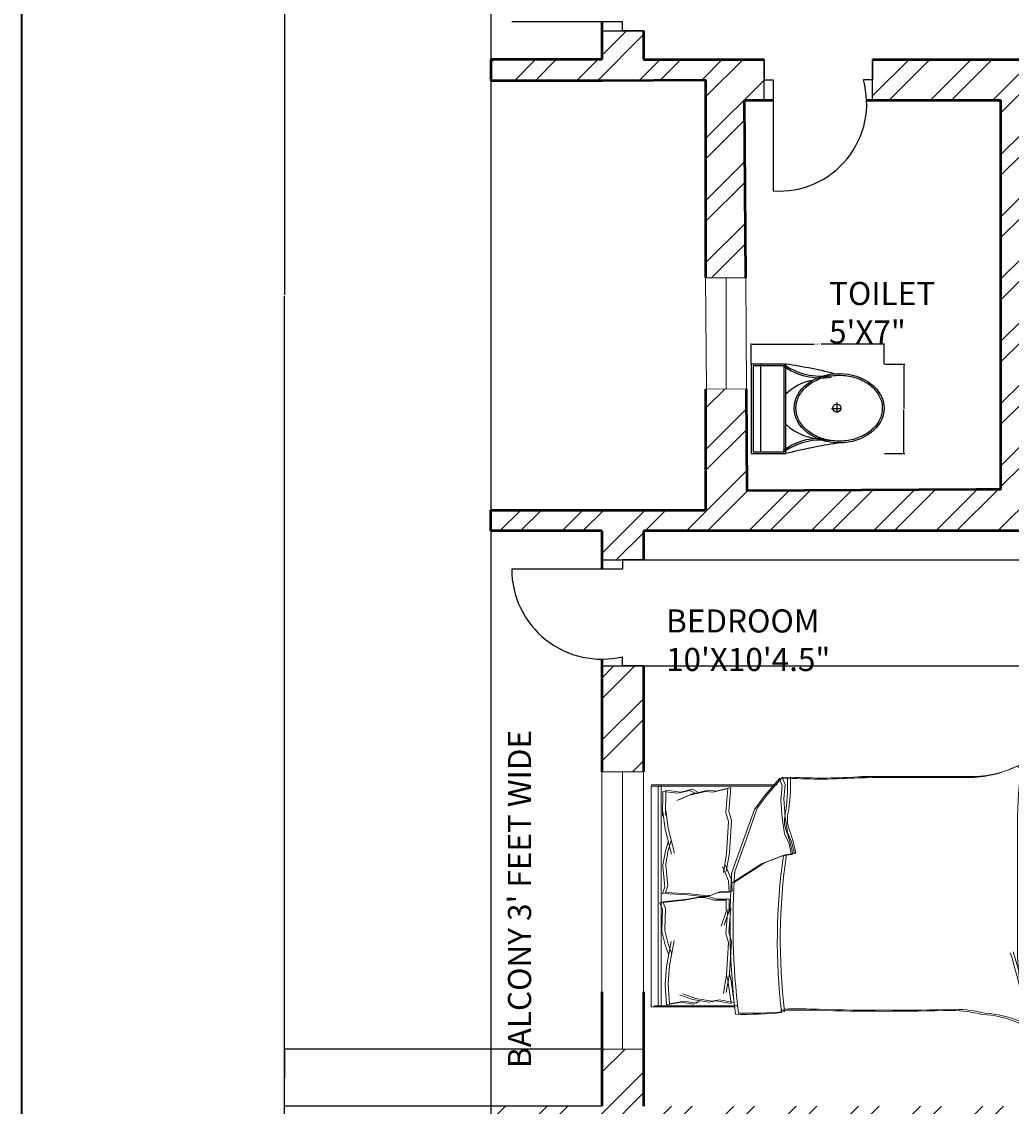
# Model space of a CAD drawing. Units: inches. Extents: x 1980 to 2738, y 1471 to 2568.
# Tile 7 of 22: x 1980 to 2194, y 1878 to 2112. Entities that reach past the tile are written whole.
import ezdxf

# ---------------------------------------------------------------- set-up
doc = ezdxf.new("R2010")
doc.units = ezdxf.units.IN
for name, color, linetype, lineweight in [('A-ANNO-DIMS', 2, 'Continuous', 18), ('A-ANNO-TTLB', 7, 'Continuous', 35), ('A-AREA-IDEN', 7, 'Continuous', 18), ('A-DOOR', 31, 'Continuous', 25), ('A-FLOR-BALC', 7, 'Continuous', 25), ('A-FLOR-FIXT', 8, 'Continuous', 25), ('A-FURN', 8, 'Continuous', 18), ('A-GLAZ', 141, 'Continuous', 18), ('A-WALL', 7, 'Continuous', 50)]:
    doc.layers.add(name, color=color, linetype=linetype, lineweight=lineweight)
doc.layers.add('A-WALL-PATT', color=9, linetype='Continuous', lineweight=13, true_color=0xd19cc7)
doc.styles.get("Standard").update_dxf_attribs({"font": 'arial.ttf'})
doc.dimstyles.get("Standard").update_dxf_attribs({"dimtxt": 0.18, "dimasz": 0.18, "dimexe": 0.18, "dimexo": 0.0625, "dimgap": 0.09, "dimtad": 0, "dimtih": 1, "dimtoh": 1, "dimdec": 4, "dimzin": 0, "dimdsep": 46, "dimtxsty": 'Standard', "dimcen": 0.09, "dimadec": 0, "dimazin": 0, "dimtfac": 1, "dimtdec": 4, "dimtofl": 0, "dimtmove": 0, "dimatfit": 3, "dimfxl": 1, "dimtolj": 1, "dimtzin": 0, "dimarcsym": 0})

# ---------------------------------------------------------------- blocks, each defined once
blk = doc.blocks.new('A$C31115884')
for p, q in [((257.5, 466.4), (257.5, 523.2)), ((283.1, 497.7), (223.4, 497.7)), ((0, 200), (0, 0)), ((520, 200), (0, 200)), ((10, 190), (10, 10)), ((510, 190), (10, 190)), ((510, 10), (510, 190)), ((520, 0), (520, 200)), ((510, 54.5), (0, 54.5)), ((10, 10), (510, 10)), ((0, 0), (520, 0))]:
    blk.add_line(p, q)
blk.add_circle((255.6, 496.4), 23.6)
for centre, radius, start, end in [((2777.7, -204.6), 2807, 165.4549, 171.71327), ((-294.5, 403.3), 364.7, 324.20913, 9.34987), ((-294.5, 403.3), 374.7, 324.20913, 9.34987), ((805.8, 403.3), 364.7, 170.65013, 215.79087), ((3237, 905), 2807, 188.28673, 194.5451), ((139.5, 406.2), 293.5, 315.84364, 2.65635), ((805.8, 403.3), 374.7, 179.20365, 215.79087), ((383.6, 406.2), 293.5, 190.27735, 224.15636)]:
    blk.add_arc(centre, radius, start, end)
blk.add_ellipse((256.2, 509.9), major_axis=(0, -260.7), ratio=0.772727)
blk.add_open_spline([(256.2, 259.2), (263.1, 259.2), (270, 259.7), (287.8, 262.3), (298.7, 265.1), (319.9, 273.1), (330.2, 278.4), (350.1, 291.1), (359.7, 298.7), (377.7, 315.9), (386.2, 325.5), (401.7, 346.6), (408.8, 358.1), (421.3, 382.5), (426.8, 395.5), (435.9, 422.4), (439.5, 436.4), (444.8, 465.1), (446.5, 479.7), (447.9, 509.2), (447.6, 524), (445, 553.3), (442.7, 567.8), (436.3, 596), (432.1, 609.7), (421.9, 636), (416, 648.6), (402.5, 672.1), (395, 683), (378.6, 703), (369.8, 712.1), (351.1, 728), (341.3, 734.8), (320.9, 746.2), (310.4, 750.7), (288.9, 757.3), (278, 759.4), (256, 761), (245, 760.6), (223.1, 757.2), (212.3, 754.3), (191.1, 746.1), (180.8, 740.7), (160.9, 727.8), (151.4, 720.1), (133.5, 702.7), (125.1, 693), (109.6, 671.7), (102.6, 660.2), (90.2, 635.7), (84.9, 622.7), (76, 595.6), (72.4, 581.6), (67.2, 552.9), (65.6, 538.2), (64.4, 508.8), (64.8, 494), (67.5, 464.7), (69.9, 450.2), (76.6, 422), (80.8, 408.3), (91.1, 382.2), (97.2, 369.7), (110.8, 346.3), (118.4, 335.4), (134.8, 315.6), (143.7, 306.7), (162.4, 290.9), (172.3, 284.2), (192.8, 273), (203.3, 268.6), (224.8, 262.2), (235.8, 260.2), (249.9, 259.3), (253, 259.2), (256.2, 259.2)], degree=3, knots=[0, 0, 0, 0, 0.110105, 0.110105, 0.285049, 0.285049, 0.459994, 0.459994, 0.634938, 0.634938, 0.809882, 0.809882, 0.984827, 0.984827, 1.159771, 1.159771, 1.334715, 1.334715, 1.50966, 1.50966, 1.684604, 1.684604, 1.859549, 1.859549, 2.034493, 2.034493, 2.209437, 2.209437, 2.384382, 2.384382, 2.559326, 2.559326, 2.73427, 2.73427, 2.909215, 2.909215, 3.084159, 3.084159, 3.259103, 3.259103, 3.434048, 3.434048, 3.608992, 3.608992, 3.783936, 3.783936, 3.958881, 3.958881, 4.133825, 4.133825, 4.30877, 4.30877, 4.483714, 4.483714, 4.658658, 4.658658, 4.833603, 4.833603, 5.008547, 5.008547, 5.183491, 5.183491, 5.358436, 5.358436, 5.53338, 5.53338, 5.708324, 5.708324, 5.883269, 5.883269, 6.058213, 6.058213, 6.233158, 6.233158, 6.283185, 6.283185, 6.283185, 6.283185])
blk = doc.blocks.new('BED-DOUBLE')
for p, q in [((27.75, 52.87), (24.5, 49.16)), ((27.75, 52.87), (24.5, 49.16)), ((28.38, 53.1), (25.13, 49.39)), ((28.38, 53.1), (25.13, 49.39)), ((29.49, 52.95), (27.75, 52.87, 3.87)), ((29.49, 52.95), (27.75, 52.87, 3.87)), ((28.36, 51.33), (27.75, 52.87)), ((28.36, 51.33), (27.75, 52.87)), ((30.13, 53.18), (28.38, 53.1, 3.87)), ((30.13, 53.18), (28.38, 53.1, 3.87)), ((29, 51.56), (28.38, 53.1)), ((29, 51.56), (28.38, 53.1)), ((0, 51.49), (0.64, 51.49)), ((0, 51.27), (26.61, 51.27)), ((0, 51.27), (26.61, 51.27)), ((0, 51.27), (0, 3.48)), ((0.64, 51.49), (27.25, 51.49)), ((0.64, 51.49), (27.25, 51.49)), ((1.53, 3.48), (1.53, 51.27)), ((1.53, 3.48), (1.53, 51.27)), ((2.17, 3.7), (2.17, 51.49)), ((2.17, 3.7), (2.17, 51.49)), ((2.56, 50.11), (2.46, 44.71)), ((2.56, 50.11), (2.46, 44.71)), ((2.56, 50.11), (5.77, 49.73)), ((2.56, 50.11), (5.77, 49.73)), ((3.2, 50.34), (3.1, 44.94)), ((3.2, 50.34), (3.1, 44.94)), ((3.2, 50.34), (6.41, 49.96)), ((3.2, 50.34), (6.41, 49.96)), ((8.26, 49.31), (5.58, 48.13)), ((8.26, 49.31), (5.58, 48.13)), ((5.77, 49.73), (8.34, 50.33)), ((5.77, 49.73), (8.34, 50.33)), ((8.9, 49.54), (6.22, 48.36)), ((8.9, 49.54), (6.22, 48.36)), ((6.41, 49.96), (8.98, 50.56)), ((6.41, 49.96), (8.98, 50.56)), ((11.83, 50.11), (8.26, 49.31)), ((11.83, 50.11), (8.26, 49.31)), ((8.34, 50.33), (9.38, 49.81)), ((8.34, 50.33), (9.38, 49.81)), ((12.47, 50.34), (8.9, 49.54)), ((12.47, 50.34), (8.9, 49.54)), ((8.98, 50.56), (10.02, 50.04)), ((8.98, 50.56), (10.02, 50.04)), ((13.43, 49.92), (11.83, 50.11)), ((13.43, 49.92), (11.83, 50.11)), ((14.07, 50.15), (12.47, 50.34)), ((14.07, 50.15), (12.47, 50.34)), ((16.57, 50.7), (13.43, 49.92)), ((16.57, 50.7), (13.43, 49.92)), ((17.21, 50.93), (14.07, 50.15)), ((17.21, 50.93), (14.07, 50.15)), ((16.17, 45.57), (16.57, 50.7)), ((16.17, 45.57), (16.57, 50.7)), ((16.81, 45.8), (17.21, 50.93)), ((16.81, 45.79), (17.21, 50.93)), ((25.13, 49.39), (22.97, 46.45)), ((25.13, 49.39), (22.97, 46.45)), ((28.06, 48.23), (28.36, 51.33)), ((28.06, 48.23), (28.36, 51.33)), ((28.69, 48.46), (29, 51.56)), ((28.69, 48.46), (29, 51.56)), ((24.5, 49.16), (22.33, 46.22)), ((24.5, 49.16), (22.33, 46.22)), ((28.36, 44.36), (28.06, 48.23)), ((28.36, 44.36), (28.06, 48.23)), ((29, 44.59), (28.69, 48.46)), ((29, 44.59), (28.69, 48.46)), ((2.46, 44.71), (2.54, 45.71)), ((2.46, 44.71), (2.54, 45.71)), ((2.54, 45.71), (3.07, 41.91)), ((2.54, 45.71), (3.07, 41.91)), ((3.1, 44.94), (3.18, 45.94)), ((3.1, 44.94), (3.18, 45.94)), ((3.18, 45.94), (3.71, 42.14)), ((3.18, 45.94), (3.71, 42.14)), ((16.73, 43.61), (16.17, 45.57)), ((16.73, 43.61), (16.17, 45.57)), ((17.37, 43.83), (16.81, 45.8)), ((17.37, 43.83), (16.81, 45.79)), ((22.33, 46.22), (20.32, 40.64)), ((22.33, 46.22), (20.32, 40.64)), ((22.97, 46.45), (20.96, 40.87)), ((22.97, 46.45), (20.96, 40.87)), ((16.29, 36.6), (16.73, 43.61)), ((16.29, 36.6), (16.73, 43.61)), ((16.93, 36.82), (17.37, 43.83)), ((16.93, 36.82), (17.37, 43.83)), ((28.83, 40.95), (28.36, 44.36)), ((28.83, 40.95), (28.36, 44.36)), ((29.47, 41.18), (29, 44.59)), ((29.47, 41.18), (29, 44.59)), ((3.07, 41.91), (4.42, 36.5)), ((3.07, 41.91), (4.42, 36.5)), ((3.71, 42.14), (5.06, 36.72)), ((3.71, 42.14), (5.06, 36.72)), ((20.32, 40.64), (17.38, 32.31)), ((20.32, 40.64), (17.38, 32.31)), ((20.96, 40.87), (18.02, 32.53)), ((20.96, 40.87), (18.02, 32.53)), ((29.76, 38.94), (28.83, 40.95)), ((29.76, 38.94), (28.83, 40.95)), ((30.4, 39.17), (29.47, 41.18)), ((30.4, 39.17), (29.47, 41.18)), ((79.88, 15.29), (79.88, 39.91)), ((79.88, 15.29), (79.88, 39.91)), ((3.67, 39.2), (3.08, 37.14)), ((3.67, 39.2), (3.08, 37.14)), ((4.31, 39.43), (3.72, 37.36)), ((4.31, 39.43), (3.72, 37.36)), ((30.38, 36.46), (29.76, 38.94)), ((30.38, 36.46), (29.76, 38.94)), ((31.02, 36.69), (30.4, 39.17)), ((31.02, 36.69), (30.4, 39.17)), ((79.24, 15.06), (79.24, 39.68)), ((79.24, 15.06), (79.24, 39.68)), ((3.08, 37.14), (2.54, 34.2)), ((3.08, 37.14), (2.54, 34.2)), ((3.72, 37.36), (3.18, 34.43)), ((3.72, 37.36), (3.18, 34.43)), ((15.63, 32.56), (16.29, 36.6)), ((15.63, 32.56), (16.29, 36.6)), ((16.27, 32.79), (16.93, 36.82)), ((16.27, 32.79), (16.93, 36.82)), ((23.88, 34.45), (28.36, 36.15)), ((23.88, 34.45), (28.36, 36.15)), ((24.52, 34.68), (29, 36.38)), ((24.52, 34.68), (29, 36.38)), ((28.36, 36.15), (30.38, 36.46)), ((28.36, 36.15), (30.38, 36.46)), ((29, 36.38), (31.02, 36.69)), ((29, 36.38), (31.02, 36.69)), ((2.54, 34.2), (2.56, 33.88)), ((2.54, 34.2), (2.56, 33.88)), ((2.56, 33.88), (2.98, 29.46)), ((2.56, 33.88), (2.98, 29.46)), ((3.18, 34.43), (3.2, 34.11)), ((3.18, 34.43), (3.2, 34.11)), ((3.2, 34.11), (3.62, 29.68)), ((3.2, 34.11), (3.62, 29.68)), ((16.74, 30.75), (15.45, 33.82)), ((16.74, 30.75), (15.45, 33.82)), ((17.38, 30.98), (16.09, 34.05)), ((17.38, 30.98), (16.09, 34.05)), ((17.38, 30.26), (23.88, 34.45)), ((17.38, 30.26), (23.88, 34.45)), ((18.02, 30.49), (24.52, 34.68)), ((18.02, 30.49), (24.52, 34.68)), ((16.89, 28.3), (16.74, 30.75)), ((16.89, 28.3), (16.74, 30.75)), ((17.53, 28.53), (17.38, 30.98)), ((17.53, 28.53), (17.38, 30.98)), ((2.98, 29.46), (2.49, 27.98)), ((2.98, 29.46), (2.49, 27.98)), ((3.62, 29.68), (3.13, 28.21)), ((3.62, 29.68), (3.13, 28.21)), ((3.13, 28.21), (8.51, 27.96)), ((3.13, 28.21), (8.51, 27.96)), ((13.02, 27.66), (14.86, 28.36)), ((13.02, 27.66), (14.86, 28.36)), ((14.22, 28.13), (16.89, 28.3)), ((14.22, 28.13), (16.89, 28.3)), ((14.86, 28.36), (17.53, 28.53)), ((14.86, 28.36), (17.53, 28.53)), ((1.87, 25.98), (7.22, 26.56)), ((1.87, 25.98), (7.22, 26.56)), ((2.45, 24.54), (1.87, 25.98)), ((2.45, 24.54), (1.87, 25.98)), ((2.49, 27.98), (7.87, 27.73)), ((2.49, 27.98), (7.87, 27.73)), ((2.51, 26.21), (7.86, 26.79)), ((2.51, 26.21), (7.86, 26.79)), ((3.09, 24.77), (2.51, 26.21)), ((3.09, 24.77), (2.51, 26.21)), ((7.22, 26.56), (10.4, 27.14)), ((7.22, 26.56), (10.4, 27.14)), ((7.86, 26.79), (11.04, 27.37)), ((7.86, 26.79), (11.04, 27.37)), ((7.87, 27.73), (11.08, 27.36)), ((7.87, 27.73), (11.08, 27.35)), ((8.51, 27.96), (11.72, 27.58)), ((8.51, 27.96), (11.72, 27.58)), ((10.4, 27.14), (11.7, 27.14)), ((10.4, 27.14), (11.7, 27.14)), ((11.04, 27.37), (12.34, 27.37)), ((11.04, 27.37), (12.34, 27.37)), ((11.08, 27.36), (12.38, 27.44)), ((11.08, 27.35), (12.38, 27.44)), ((11.7, 27.14), (13.58, 26.56)), ((11.7, 27.14), (13.58, 26.56)), ((11.72, 27.58), (13.02, 27.66)), ((11.72, 27.58), (13.02, 27.66)), ((12.34, 27.37), (14.22, 26.79)), ((12.34, 27.37), (14.22, 26.79)), ((12.38, 27.44), (14.22, 28.13)), ((12.38, 27.44), (14.22, 28.13)), ((13.58, 26.56), (16.26, 26.56)), ((13.58, 26.56), (16.26, 26.56)), ((14.22, 26.79), (16.9, 26.79)), ((14.22, 26.79), (16.9, 26.79)), ((16.26, 26.56), (16.26, 24.1)), ((16.26, 26.56), (16.26, 24.1)), ((16.9, 26.79), (16.9, 24.33)), ((16.9, 26.79), (16.9, 24.33)), ((2.3, 20.09), (2.45, 24.54)), ((2.3, 20.09), (2.45, 24.54)), ((2.94, 20.32), (3.09, 24.77)), ((2.94, 20.32), (3.09, 24.77)), ((16.26, 24.1), (15.17, 20.96)), ((16.26, 24.1), (15.17, 20.96)), ((16.9, 24.33), (15.81, 21.19)), ((16.9, 24.33), (15.81, 21.19)), ((16.17, 19.38), (16.57, 24.52)), ((16.17, 19.38), (16.57, 24.52)), ((16.81, 19.61), (17.21, 24.74)), ((16.81, 19.61), (17.21, 24.74)), ((2.3, 19.77), (2.3, 20.09)), ((2.3, 19.77), (2.3, 20.09)), ((3.03, 16.88), (2.3, 19.77)), ((3.03, 16.88), (2.3, 19.77)), ((2.94, 20), (2.94, 20.32)), ((2.94, 20), (2.94, 20.32)), ((3.67, 17.11), (2.94, 20)), ((3.67, 17.11), (2.94, 20)), ((16.73, 17.42), (16.17, 19.38)), ((16.73, 17.42), (16.17, 19.38)), ((17.37, 17.65), (16.81, 19.61)), ((17.37, 17.65), (16.81, 19.61)), ((3.75, 14.86), (3.03, 16.88)), ((3.75, 14.85), (3.03, 16.88)), ((3.32, 12.11), (4.33, 17.6)), ((3.32, 12.11), (4.33, 17.6)), ((4.39, 15.08), (3.67, 17.11)), ((4.39, 15.08), (3.67, 17.11)), ((3.96, 12.34), (4.97, 17.83)), ((3.96, 12.34), (4.97, 17.83)), ((16.29, 10.41), (16.73, 17.42)), ((16.29, 10.41), (16.73, 17.42)), ((16.93, 10.64), (17.37, 17.65)), ((16.93, 10.64), (17.37, 17.65)), ((3.03, 8.29), (3.32, 12.11)), ((3.03, 8.28), (3.32, 12.11)), ((3.67, 8.51), (3.96, 12.34)), ((3.67, 8.51), (3.96, 12.34)), ((15.63, 6.38), (16.29, 10.41)), ((15.63, 6.38), (16.29, 10.41)), ((16.27, 6.61), (16.93, 10.64)), ((16.27, 6.61), (16.93, 10.64)), ((16.29, 10.41), (16.62, 9.28)), ((16.29, 10.41), (16.62, 9.28)), ((16.93, 10.64), (17.26, 9.51)), ((16.93, 10.64), (17.26, 9.51)), ((17.26, 9.51), (17.98, 4.41)), ((17.26, 9.51), (17.98, 4.41)), ((3.01, 8.18), (3.03, 8.29)), ((3.01, 8.18), (3.03, 8.28)), ((3.34, 3.9), (3.01, 8.18)), ((3.34, 3.9), (3.01, 8.18)), ((3.65, 8.41), (3.67, 8.51)), ((3.65, 8.41), (3.67, 8.51)), ((3.98, 4.13), (3.65, 8.41)), ((3.98, 4.13), (3.65, 8.41)), ((16.62, 9.28), (17.34, 4.18)), ((16.62, 9.28), (17.34, 4.18)), ((3.96, 4.12), (7.14, 4.7)), ((3.96, 4.12), (7.14, 4.7)), ((8.95, 5.05), (6.21, 6.06)), ((8.95, 5.05), (6.21, 6.06)), ((9.59, 5.28), (6.85, 6.29)), ((9.59, 5.28), (6.85, 6.29)), ((7.14, 4.7), (9.74, 4.27)), ((7.14, 4.7), (9.74, 4.27)), ((12.57, 4.47), (8.95, 5.05)), ((12.57, 4.47), (8.95, 5.05)), ((13.21, 4.7), (9.59, 5.28)), ((13.21, 4.7), (9.59, 5.28)), ((9.74, 4.27), (10.75, 4.85)), ((9.74, 4.27), (10.75, 4.85)), ((14.16, 4.76), (12.57, 4.47)), ((14.16, 4.76), (12.57, 4.47)), ((14.8, 4.99), (13.21, 4.7)), ((14.8, 4.99), (13.21, 4.7)), ((17.34, 4.18), (14.16, 4.76)), ((17.34, 4.18), (14.16, 4.76)), ((17.98, 4.41), (14.8, 4.99)), ((17.98, 4.41), (14.8, 4.99)), ((18.11, 3.48), (0, 3.48)), ((18.11, 3.48), (0, 3.48)), ((18.75, 3.7), (0.64, 3.7)), ((18.75, 3.7), (0.64, 3.7)), ((3.32, 3.89), (6.5, 4.47)), ((3.32, 3.89), (6.5, 4.47)), ((6.5, 4.47), (9.1, 4.04)), ((6.5, 4.47), (9.1, 4.04)), ((9.1, 4.04), (10.11, 4.62)), ((9.1, 4.04), (10.11, 4.62))]:
    blk.add_line(p, q)
for centre, radius, start, end in [((68.67, 76.16), 23.07, 267.4714, 296.4681), ((68.67, 76.16), 23.07, 267.4714, 296.4681), ((69.31, 76.39), 23.07, 267.4714, 296.4681), ((69.31, 76.39), 23.07, 267.4714, 296.4681), ((78.87, 54.41), 1.1, 332.6588, 86.02), ((78.87, 54.41), 1.1, 332.6588, 86.02), ((79.51, 54.64), 1.1, 332.6588, 86.02), ((79.51, 54.64), 1.1, 332.6588, 86.02), ((212.92, 41.38), 133.04, 174.4998, 180.6351), ((212.92, 41.38), 133.04, 174.4998, 180.6351), ((-6.66, 51.33), 36.18, 349.8763, 2.5657), ((-6.66, 51.33), 36.18, 349.8763, 2.5657), ((36.31, 182.27), 129.5, 266.9791, 273.8365), ((36.31, 182.27), 129.5, 266.9791, 273.8365), ((-6.02, 51.56), 36.18, 349.8763, 2.5657), ((-6.02, 51.56), 36.18, 349.8763, 2.5657), ((36.95, 182.49), 129.5, 266.9791, 273.8365), ((36.95, 182.49), 129.5, 266.9791, 273.8365), ((67.82, -4508.74), 4561.86, 90.00217, 90.28689), ((67.82, -4508.74), 4561.86, 90.00217, 90.28689), ((68.46, -4508.51), 4561.86, 90.00217, 90.28689), ((68.46, -4508.52), 4561.86, 90.00217, 90.28689), ((212.28, 41.15), 133.04, 174.4998, 180.6351), ((212.28, 41.15), 133.04, 174.4998, 180.6351), ((35.07, 43.74), 6.22, 168.6608, 203.7384), ((35.07, 43.74), 6.22, 168.6608, 203.7384), ((35.71, 43.97), 6.22, 168.6608, 203.7384), ((35.71, 43.97), 6.22, 168.6608, 203.7384), ((1.48, 31.15), 29.65, 10.6617, 19.8806), ((1.48, 31.15), 29.65, 10.6617, 19.8806), ((2.12, 31.38), 29.65, 10.6617, 19.8806), ((2.12, 31.38), 29.65, 10.6617, 19.8806), ((156.32, 17.76), 129.02, 171.7845, 186.9006), ((156.32, 17.76), 129.02, 171.7845, 186.9006), ((156.96, 17.98), 129.02, 171.7845, 186.9006), ((156.96, 17.98), 129.02, 171.7845, 186.9006), ((30.44, 36.64), 0.185, 250.2464, 1.1377), ((30.44, 36.64), 0.185, 250.2464, 1.1377), ((31.08, 36.86), 0.185, 250.2464, 1.1377), ((31.08, 36.86), 0.185, 250.2464, 1.1377), ((182.05, 21.36), 164.97, 176.0865, 186.7821), ((182.05, 21.36), 164.97, 176.0865, 186.7821), ((182.69, 21.59), 164.97, 176.0865, 186.7821), ((182.69, 21.59), 164.97, 176.0865, 186.7821), ((-23.71, -17.22), 106.46, 13.3832, 17.7053), ((-23.71, -17.22), 106.46, 13.3832, 17.7053), ((-23.07, -16.99), 106.46, 13.3832, 17.7053), ((-23.07, -16.99), 106.46, 13.3832, 17.7053), ((200.84, 21.43), 121.76, 182.9958, 189.4091), ((200.84, 21.43), 121.76, 182.9958, 189.4091), ((201.48, 21.66), 121.76, 182.9958, 189.4091), ((201.48, 21.66), 121.76, 182.9958, 189.4091), ((20.74, 85.39), 83.31, 268.7218, 275.604), ((20.74, 85.39), 83.31, 268.7218, 275.604), ((31.17, -167.31), 170.11, 88.4762, 91.0082), ((31.17, -167.31), 170.11, 88.4762, 91.0082), ((31.81, -167.08), 170.11, 88.4762, 91.0082), ((31.81, -167.08), 170.11, 88.4762, 91.0082), ((50.61, 484.82), 482.31, 268.2277, 271.7185), ((50.61, 484.82), 482.31, 268.2277, 271.7185), ((51.25, 485.05), 482.31, 268.2277, 271.7185), ((51.25, 485.05), 482.31, 268.2277, 271.7185), ((64.51, -26.9), 29.63, 76.0648, 88.9113), ((64.51, -26.9), 29.63, 76.0648, 88.9113), ((65.15, -26.67), 29.63, 76.0648, 88.9113), ((65.15, -26.67), 29.63, 76.0648, 88.9113), ((20.1, 85.16), 83.31, 268.7218, 275.604), ((20.1, 85.16), 83.31, 268.7218, 275.604), ((70.28, -21.66), 23.56, 67.9751, 86.652), ((70.28, -21.66), 23.56, 67.9751, 86.652), ((70.91, -21.43), 23.56, 67.9751, 86.652), ((70.91, -21.43), 23.56, 67.9751, 86.652), ((79.72, 1.09), 1.09, 236.1736, 23.4781), ((79.72, 1.09), 1.09, 236.1736, 23.4781), ((80.36, 1.32), 1.09, 236.1736, 23.4781), ((80.36, 1.32), 1.09, 236.1736, 23.4781)]:
    blk.add_arc(centre, radius, start, end)
blk = doc.blocks.new('WIN-60IN-WALL-SINGLE-JAMB-LINE')
for p, q in [((4.5, 60), (0, 60)), ((0, 60), (9, 60)), ((0, 60), (0, 0)), ((4.5, 0), (4.5, 60)), ((9, 60), (9, 0)), ((0, 0), (9, 0))]:
    blk.add_line(p, q)
blk = doc.blocks.new('*D13')
at = {"layer": 'A-ANNO-DIMS', "color": 0, "lineweight": -2, "transparency": 16777216}
for p, q in [((2137.43, 2038.37), (2137.43, 2042.8)), ((2137.61, 2042.62), (2151.01, 2042.62)), ((2165.97, 2042.62), (2152.56, 2042.62)), ((2166.15, 2038.37), (2166.15, 2042.8))]:
    blk.add_line(p, q, dxfattribs=at)
at = {"layer": 'A-ANNO-DIMS', "color": 0, "transparency": 16777216}
for points in [[(2137.61, 2042.65), (2137.61, 2042.59), (2137.43, 2042.62)], [(2165.97, 2042.65), (2165.97, 2042.59), (2166.15, 2042.62)]]:
    blk.add_solid(points, dxfattribs=at)
at = {"layer": 'Defpoints', "color": 0, "transparency": 16777216}
for p in [(2166.15, 2042.62), (2137.43, 2038.31), (2166.15, 2038.31)]:
    blk.add_point(p, dxfattribs=at)
at = {"layer": 'A-ANNO-DIMS', "color": 0, "transparency": 16777216, "insert": (2151.79, 2042.62), "char_height": 0.18, "attachment_point": 5}
blk.add_mtext('\\A1;WC 29 TYP.', dxfattribs=at)
blk = doc.blocks.new('*D14')
at = {"layer": 'A-ANNO-DIMS', "color": 0, "lineweight": -2, "transparency": 16777216}
for p, q in [((2166.21, 2038.31), (2170.64, 2038.31)), ((2170.46, 2038.13), (2170.46, 2028.8)), ((2170.46, 2019.11), (2170.46, 2028.44)), ((2166.21, 2018.93), (2170.64, 2018.93))]:
    blk.add_line(p, q, dxfattribs=at)
at = {"layer": 'A-ANNO-DIMS', "color": 0, "transparency": 16777216}
for points in [[(2170.43, 2038.13), (2170.49, 2038.13), (2170.46, 2038.31)], [(2170.43, 2019.11), (2170.49, 2019.11), (2170.46, 2018.93)]]:
    blk.add_solid(points, dxfattribs=at)
at = {"layer": 'Defpoints', "color": 0, "transparency": 16777216}
for p in [(2166.15, 2038.31), (2166.15, 2018.93), (2170.46, 2018.93)]:
    blk.add_point(p, dxfattribs=at)
at = {"layer": 'A-ANNO-DIMS', "color": 0, "transparency": 16777216, "insert": (2170.46, 2028.62), "char_height": 0.18, "attachment_point": 5}
blk.add_mtext('\\A1;19 TYP.', dxfattribs=at)
blk = doc.blocks.new('*D36')
at = {"layer": 'A-ANNO-DIMS', "color": 0, "lineweight": -2, "transparency": 16777216}
for p, q in [((2105.02, 2462.71), (2036.25, 2462.71)), ((2036.43, 2462.53), (2036.43, 2053.39)), ((2036.43, 1643.89), (2036.43, 2053.02)), ((2105.02, 1643.71), (2036.25, 1643.71))]:
    blk.add_line(p, q, dxfattribs=at)
at = {"layer": 'A-ANNO-DIMS', "color": 0, "transparency": 16777216}
for points in [[(2036.4, 2462.53), (2036.46, 2462.53), (2036.43, 2462.71)], [(2036.4, 1643.89), (2036.46, 1643.89), (2036.43, 1643.71)]]:
    blk.add_solid(points, dxfattribs=at)
at = {"layer": 'Defpoints', "color": 0, "transparency": 16777216}
for p in [(2036.43, 2462.71), (2105.08, 2462.71), (2105.08, 1643.71)]:
    blk.add_point(p, dxfattribs=at)
at = {"layer": 'A-ANNO-DIMS', "color": 0, "transparency": 16777216, "insert": (2036.43, 2053.21), "char_height": 0.18, "attachment_point": 5}
blk.add_mtext('\\A1;819', dxfattribs=at)
blk = doc.blocks.new('*D56')
at = {"layer": 'A-ANNO-DIMS', "color": 0, "lineweight": -2, "transparency": 16777216}
for p, q in [((2114.15, 1995.93), (2689.91, 1995.93)), ((2689.73, 1995.75), (2689.73, 1984.65)), ((2689.73, 1973.18), (2689.73, 1984.28)), ((2114.15, 1973), (2689.91, 1973))]:
    blk.add_line(p, q, dxfattribs=at)
at = {"layer": 'A-ANNO-DIMS', "color": 0, "transparency": 16777216}
for points in [[(2689.7, 1995.75), (2689.76, 1995.75), (2689.73, 1995.93)], [(2689.7, 1973.18), (2689.76, 1973.18), (2689.73, 1973)]]:
    blk.add_solid(points, dxfattribs=at)
at = {"layer": 'Defpoints', "color": 0, "transparency": 16777216}
for p in [(2114.08, 1995.93), (2689.73, 1995.93), (2114.08, 1973)]:
    blk.add_point(p, dxfattribs=at)
at = {"layer": 'A-ANNO-DIMS', "color": 0, "transparency": 16777216, "insert": (2689.73, 1984.47), "char_height": 0.18, "attachment_point": 5}
blk.add_mtext('\\A1;22.935', dxfattribs=at)
blk = doc.blocks.new('*D62')
at = {"layer": 'A-ANNO-DIMS', "color": 0, "lineweight": -2, "transparency": 16777216}
for p, q in [((2105.02, 1890.1), (2036.25, 1890.1)), ((2036.43, 1889.92), (2036.43, 1884.08)), ((2036.43, 1877.89), (2036.43, 1883.72)), ((2105.02, 1877.71), (2036.25, 1877.71))]:
    blk.add_line(p, q, dxfattribs=at)
at = {"layer": 'A-ANNO-DIMS', "color": 0, "transparency": 16777216}
for points in [[(2036.4, 1889.92), (2036.46, 1889.92), (2036.43, 1890.1)], [(2036.4, 1877.89), (2036.46, 1877.89), (2036.43, 1877.71)]]:
    blk.add_solid(points, dxfattribs=at)
at = {"layer": 'Defpoints', "color": 0, "transparency": 16777216}
for p in [(2036.43, 1890.1), (2105.08, 1890.1), (2105.08, 1877.71)]:
    blk.add_point(p, dxfattribs=at)
at = {"layer": 'A-ANNO-DIMS', "color": 0, "transparency": 16777216, "insert": (2036.43, 1883.9), "char_height": 0.18, "attachment_point": 5}
blk.add_mtext('\\A1;12.39', dxfattribs=at)

msp = doc.modelspace()

# ---------------------------------------------------------------- hatches: boundary and pattern name
at = {"layer": 'A-WALL-PATT'}
h = msp.add_hatch(dxfattribs=at)
h.set_pattern_fill('ANSI32', color=256)
h.paths.add_polyline_path([(2257.5661, 2416.2064), (2257.5661, 2420.7064), (2250.5833, 2420.7064), (2250.5833, 2462.7064), (2246.0833, 2462.7064), (2246.0833, 2420.7064), (2237.0791, 2420.7064), (2237.0791, 2411.7064), (2246.0833, 2411.7064), (2246.0833, 2291.7064), (2242.6109, 2291.7064), (2242.6109, 2287.2064), (2246.0833, 2287.2064), (2250.5833, 2287.2064), (2250.5833, 2291.7064), (2250.5833, 2411.7064), (2257.5661, 2411.7064)])
h.paths.add_polyline_path([(2387.0396, 2416.2064), (2387.0396, 2420.7064), (2367.5833, 2420.7064), (2367.5833, 2462.7064), (2358.5833, 2462.7064), (2358.5833, 2420.7064), (2329.3087, 2420.7064), (2329.3087, 2411.7064), (2358.5833, 2411.7064), (2358.5833, 2321.7275), (2358.5833, 2309.7064), (2347.3089, 2309.7064), (2293.3089, 2309.7064), (2293.3089, 2259.0771), (2297.8089, 2259.0771), (2297.8089, 2305.2064), (2347.3089, 2305.2064), (2347.3089, 2284.7412), (2351.8089, 2284.7412), (2351.8089, 2305.2064), (2372.3188, 2305.2064), (2372.3761, 2284.3899), (2377.0295, 2284.3899), (2377.0295, 2299.3058), (2377.0295, 2305.2064), (2426.5295, 2305.2064), (2426.5295, 2257.5573), (2431.0295, 2257.5573), (2431.0295, 2309.7064), (2377.0295, 2309.7064), (2367.5833, 2309.7064), (2367.5833, 2321.7275), (2367.5833, 2411.7064), (2387.0396, 2411.7064)])
h.paths.add_polyline_path([(2448.5267, 2416.2064), (2448.5267, 2420.7064), (2423.0396, 2420.7064), (2423.0396, 2411.7064), (2448.5267, 2411.7064)])
h.paths.add_polyline_path([(2130.9128, 2416.2064), (2130.9128, 2420.7064), (2105.0833, 2420.7064), (2105.0833, 2386.6942), (2114.0833, 2386.6942), (2114.0833, 2411.7064), (2130.9128, 2411.7064)])
h.paths.add_polyline_path([(2212.9478, 2420.7064), (2190.9128, 2420.7064), (2190.9128, 2411.7064), (2212.9478, 2411.7064), (2212.9478, 2416.2064)])
h.paths.add_polyline_path([(2114.0833, 2326.6942), (2105.0833, 2326.6942), (2105.0833, 2291.7064), (2081.0833, 2291.7064), (2081.0833, 2287.2064), (2105.0833, 2287.2064), (2105.0833, 2276.1935), (2114.0833, 2276.1935), (2114.0833, 2287.2064), (2166.3825, 2287.2064), (2166.3825, 2289.4564), (2166.3825, 2291.7064), (2114.0833, 2291.7064)])
h.paths.add_polyline_path([(2114.0833, 2252.1935), (2105.0833, 2252.1935), (2105.0833, 2233.2064), (2081.0833, 2233.2064), (2081.0833, 2228.7064), (2105.0833, 2228.7064), (2105.0833, 2213.4478), (2114.0833, 2213.4478), (2114.0833, 2228.7064), (2195.0833, 2228.7064), (2199.5833, 2228.7064), (2208.4455, 2228.7064), (2208.4455, 2230.9564), (2208.4455, 2233.2064), (2199.5833, 2233.2064), (2199.5833, 2287.2064), (2206.8904, 2287.2064), (2206.8904, 2289.4564), (2206.8904, 2291.7064), (2189.446, 2291.7064), (2189.446, 2289.4564), (2189.446, 2287.2064), (2195.0833, 2287.2064), (2195.0833, 2233.2064), (2114.0833, 2233.2064)])
h.paths.add_polyline_path([(2114.0833, 2153.4478), (2109.5833, 2153.4478), (2105.0833, 2153.4478), (2105.0833, 2135.2374), (2114.0833, 2135.2374)], flags=17)
h.paths.add_polyline_path([(2135.9619, 2095.4081), (2140.1805, 2095.4081), (2140.1805, 2104.2064), (2114.0833, 2104.2064), (2114.0833, 2110.3997), (2109.5833, 2110.3997), (2105.0833, 2110.3997), (2105.0833, 2104.2064), (2081.0833, 2104.2064), (2081.0833, 2099.7064), (2105.0833, 2099.7064), (2127.5416, 2099.8532), (2127.5416, 2056.9393), (2136.2133, 2056.9393)], flags=17)
h.paths.add_polyline_path([(2255.4895, 2104.2064), (2250.5833, 2104.2064), (2250.5833, 2233.2064), (2246.0833, 2233.2064), (2242.4941, 2233.2064), (2242.4941, 2228.7064), (2246.0833, 2228.7064), (2246.0833, 2104.2064), (2163.6825, 2104.2064), (2163.6825, 2099.8072), (2163.6825, 2095.4081), (2191.4325, 2095.4081), (2191.4325, 2011.2064), (2186.0833, 2011.2064), (2136.5143, 2010.8824), (2136.3702, 2032.9403), (2131.9559, 2032.9115), (2127.5416, 2032.8826), (2127.5416, 2006.7064), (2105.0833, 2006.7064), (2081.0833, 2006.7064), (2081.0833, 2002.2064), (2105.0833, 2002.2064), (2105.0833, 1995.9329), (2114.0833, 1995.9329), (2114.0833, 2002.2064), (2246.0833, 2002.2064), (2246.0833, 1877.7064), (2242.1358, 1877.7064), (2242.1358, 1873.2064), (2250.5833, 1873.2064), (2250.5833, 2002.2064), (2255.3335, 2002.2064), (2255.3335, 2011.2064), (2195.9325, 2011.2064), (2195.9325, 2095.2064), (2255.4895, 2095.2064), (2255.4895, 2099.5471)])
h.paths.add_polyline_path([(2199.5833, 1873.2064), (2209.827, 1873.2064), (2209.827, 1875.4564), (2209.827, 1877.7064), (2114.0833, 1877.7064), (2114.0833, 1890.0968), (2105.0833, 1890.0968), (2105.0833, 1877.7064), (2081.0833, 1877.7064), (2081.0833, 1873.2064), (2105.0833, 1873.2064), (2105.0833, 1857.7279), (2114.0833, 1857.7279), (2114.0833, 1873.2064), (2195.0833, 1873.2064), (2195.0833, 1819.2064), (2190.298, 1819.2064), (2190.298, 1814.7064), (2209.8976, 1814.7064), (2209.8976, 1816.9564), (2209.8976, 1819.2064), (2199.5833, 1819.2064)])
h.paths.add_polyline_path([(2114.0833, 1814.7064), (2166.2538, 1814.7064), (2166.2538, 1816.9564), (2166.2538, 1819.2064), (2114.0833, 1819.2064), (2114.0833, 1833.7279), (2109.5833, 1833.7279), (2105.0833, 1833.7279), (2105.0833, 1819.2064), (2081.0833, 1819.2064), (2081.0833, 1814.7064), (2105.0833, 1814.7064), (2105.0833, 1782.5516), (2114.0833, 1782.5516)])
h.paths.add_polyline_path([(2114.0833, 1722.5516), (2109.5833, 1722.5516), (2105.0833, 1722.5516), (2105.0833, 1685.7064), (2124.5104, 1685.7064), (2124.5104, 1690.2064), (2124.5104, 1694.7064), (2114.0833, 1694.7064)])
h.paths.add_polyline_path([(2218.8787, 1694.7064), (2184.5104, 1694.7064), (2184.5104, 1685.7064), (2218.8787, 1685.7064), (2218.8787, 1690.2064)])
h.paths.add_polyline_path([(2250.5833, 1819.2064), (2242.6431, 1819.2064), (2242.6431, 1816.9564), (2242.6431, 1814.7064), (2246.0833, 1814.7064), (2246.0833, 1694.7064), (2240.4035, 1694.7064), (2240.4035, 1690.2064), (2240.4035, 1685.7064), (2246.0833, 1685.7064), (2246.0833, 1643.7064), (2250.5833, 1643.7064), (2250.5833, 1685.7064), (2255.9859, 1685.7064), (2255.9859, 1690.2064), (2255.9859, 1694.7064), (2250.5833, 1694.7064)])
h.paths.add_polyline_path([(2297.4764, 1694.7064), (2279.3934, 1694.7064), (2279.3934, 1690.2064), (2279.3934, 1685.7064), (2297.4764, 1685.7064), (2297.4764, 1690.2064)])
h.paths.add_polyline_path([(2377.1596, 1694.7064), (2367.5833, 1694.7064), (2367.5833, 1787.7064), (2431.0295, 1787.7064), (2431.0295, 1792.2064), (2431.0295, 1849.4149), (2428.7795, 1849.4149), (2426.5295, 1849.4149), (2426.5295, 1792.2064), (2421.5833, 1792.2064), (2367.5833, 1792.2064), (2297.8089, 1792.2064), (2297.8089, 1850.2946), (2295.5589, 1850.2946), (2293.3089, 1850.2946), (2293.3089, 1792.2064), (2293.3089, 1787.7064), (2297.8089, 1787.7064), (2358.5833, 1787.7064), (2358.5833, 1694.7064), (2333.4764, 1694.7064), (2333.4764, 1685.7064), (2358.5833, 1685.7064), (2358.5833, 1643.7064), (2367.5833, 1643.7064), (2367.5833, 1685.7064), (2377.1596, 1685.7064)])
h.paths.add_polyline_path([(2442.4912, 1694.7064), (2413.1596, 1694.7064), (2413.1596, 1685.7064), (2442.4912, 1685.7064)])
h.paths.add_polyline_path([(2480.0833, 1814.7064), (2483.4816, 1814.7064), (2483.4816, 1817.9384), (2483.4816, 1819.2064), (2475.5833, 1819.2064), (2475.5833, 1694.7064), (2470.7283, 1694.7064), (2470.7283, 1685.7064), (2475.5833, 1685.7064), (2475.5833, 1643.7064), (2480.0833, 1643.7064), (2480.0833, 1685.7064), (2486.3293, 1685.7064), (2486.3293, 1690.2064), (2486.3293, 1694.7064), (2480.0833, 1694.7064)])
h.paths.add_polyline_path([(2621.0833, 1721.7349), (2612.0833, 1721.7349), (2612.0833, 1694.7064), (2586.1453, 1694.7064), (2586.1453, 1685.7064), (2621.0833, 1685.7064)])
h.paths.add_polyline_path([(2526.1453, 1690.2064), (2526.1453, 1694.7064), (2511.584, 1694.7064), (2511.584, 1690.2064), (2511.584, 1685.7064), (2526.1453, 1685.7064)])
h.paths.add_polyline_path([(2645.0833, 1819.2064), (2621.0833, 1819.2064), (2621.0833, 1835.8527), (2616.5833, 1835.8527), (2612.0833, 1835.8527), (2612.0833, 1819.2064), (2560.2541, 1819.2064), (2560.2541, 1814.7064), (2612.0833, 1814.7064), (2612.0833, 1781.7349), (2621.0833, 1781.7349), (2621.0833, 1814.7064), (2645.0833, 1814.7064)])
h.paths.add_polyline_path([(2645.0833, 1877.7064), (2621.0833, 1877.7064), (2621.0833, 1886.4375), (2612.0833, 1886.4375), (2612.0833, 1877.7064), (2517.1032, 1877.7064), (2517.1032, 1875.4564), (2517.1032, 1873.2064), (2526.5833, 1873.2064), (2526.5833, 1819.2064), (2516.6454, 1819.2064), (2516.6454, 1816.9564), (2516.6454, 1814.7064), (2536.4445, 1814.7064), (2536.4445, 1816.9564), (2536.4445, 1819.2064), (2531.0833, 1819.2064), (2531.0833, 1873.2064), (2612.0833, 1873.2064), (2612.0833, 1859.8527), (2621.0833, 1859.8527), (2621.0833, 1873.2064), (2645.0833, 1873.2064)])
h.paths.add_polyline_path([(2645.0833, 2006.7064), (2621.0833, 2006.7064), (2588.5085, 2006.7064), (2588.5085, 2052.9125), (2579.9045, 2052.9125), (2579.9045, 2011.2064), (2519.9045, 2011.2064), (2519.9045, 2095.2064), (2553.1204, 2095.2064), (2553.1204, 2104.2064), (2480.0833, 2104.2064), (2480.0833, 2228.7064), (2484.3832, 2228.7064), (2484.3832, 2230.9564), (2484.3832, 2233.2064), (2475.5833, 2233.2064), (2475.5833, 2104.2064), (2463.1308, 2104.2064), (2463.1308, 2095.2064), (2501.2463, 2095.2064), (2510.9045, 2095.2064), (2515.4045, 2095.2064), (2515.4045, 2011.2064), (2510.9045, 2011.2064), (2501.2463, 2011.2064), (2462.5957, 2011.2064), (2462.5957, 2002.2064), (2475.5833, 2002.2064), (2475.5833, 1873.2064), (2483.6146, 1873.2064), (2483.6146, 1875.4564), (2483.6146, 1877.7064), (2480.0833, 1877.7064), (2480.0833, 2002.2064), (2612.0833, 2002.2064), (2612.0833, 1996.309), (2621.0833, 1996.309), (2621.0833, 2002.2064), (2645.0833, 2002.2064)])
h.paths.add_polyline_path([(2588.5085, 2099.7277), (2621.0833, 2099.7277), (2645.0833, 2099.7064), (2645.0833, 2104.2064), (2621.0833, 2104.2064), (2621.0833, 2109.0038), (2616.5833, 2109.0038), (2612.0833, 2109.0038), (2612.0833, 2104.2064), (2575.0621, 2104.2064), (2575.0621, 2099.7064), (2575.0621, 2095.2064), (2579.9045, 2095.2064), (2579.9045, 2076.9125), (2588.5085, 2076.9125)], flags=17)
h.paths.add_polyline_path([(2367.5833, 2002.2064), (2373.7228, 2002.2064), (2373.7228, 2006.7064), (2373.7228, 2011.2064), (2350.7889, 2011.2064), (2350.7889, 2006.7064), (2350.7889, 2002.2064), (2358.5833, 2002.2064), (2358.5833, 1877.7064), (2293.3089, 1877.7064), (2293.3089, 1870.4987), (2297.8089, 1870.4987), (2297.8089, 1873.2064), (2347.3089, 1873.2064), (2347.3089, 1847.2208), (2351.8089, 1847.2208), (2351.8089, 1873.2064), (2372.5295, 1873.2064), (2372.5295, 1847.8619), (2377.0295, 1847.8619), (2377.0295, 1873.2064), (2426.5295, 1873.2064), (2426.5295, 1868.7339), (2431.0295, 1868.7339), (2431.0295, 1877.7064), (2367.5833, 1877.7064)])
h.paths.add_polyline_path([(2531.0833, 2287.2064), (2534.2285, 2287.2064), (2534.2285, 2291.7064), (2516.7886, 2291.7064), (2516.7886, 2287.2064), (2526.5833, 2287.2064), (2526.5833, 2233.2064), (2517.9112, 2233.2064), (2517.9112, 2230.9564), (2517.9112, 2228.7064), (2526.5833, 2228.7064), (2531.0833, 2228.7064), (2612.0833, 2228.7064), (2612.0833, 2206.8504), (2621.0833, 2206.8504), (2621.0833, 2228.7064), (2645.0833, 2228.7064), (2645.0833, 2233.2064), (2621.0833, 2233.2064), (2621.0833, 2241.8536), (2616.5833, 2241.8536), (2612.0833, 2241.8536), (2612.0833, 2233.2064), (2531.0833, 2233.2064)])
h.paths.add_polyline_path([(2645.0833, 2291.7064), (2621.0833, 2291.7064), (2621.0833, 2323.0138), (2616.5833, 2323.0138), (2612.0833, 2323.0138), (2612.0833, 2291.7064), (2559.6852, 2291.7064), (2559.6852, 2289.4564), (2559.6852, 2287.2064), (2612.0833, 2287.2064), (2612.0833, 2265.8536), (2621.0833, 2265.8536), (2621.0833, 2287.2064), (2645.0833, 2287.2064)])
h.paths.add_polyline_path([(2621.0833, 2420.7064), (2582.8189, 2420.7064), (2582.8189, 2411.7064), (2612.0833, 2411.7064), (2612.0833, 2383.0138), (2621.0833, 2383.0138)])
h.paths.add_polyline_path([(2480.0833, 2411.7064), (2485.7342, 2411.7064), (2485.7342, 2416.2064), (2485.7342, 2420.7064), (2480.0833, 2420.7064), (2480.0833, 2462.7064), (2475.5833, 2462.7064), (2475.5833, 2420.7064), (2469.4083, 2420.7064), (2469.4083, 2411.7064), (2475.5833, 2411.7064), (2475.5833, 2291.7064), (2475.5833, 2287.2064), (2482.9195, 2287.2064), (2482.9195, 2289.4564), (2482.9195, 2291.7064), (2480.0833, 2291.7064)])
h.paths.add_polyline_path([(2367.5833, 2228.7064), (2431.0295, 2228.7064), (2431.0295, 2233.2064), (2431.0295, 2237.4203), (2428.7795, 2237.4203), (2426.5295, 2237.4203), (2426.5295, 2233.2064), (2377.0295, 2233.2064), (2377.0295, 2260.3837), (2372.4423, 2260.3837), (2372.517, 2233.2635), (2351.8089, 2233.2064), (2351.8089, 2260.7412), (2347.3089, 2260.7412), (2347.3089, 2233.2064), (2297.8089, 2233.2064), (2297.8089, 2236.9324), (2293.3089, 2236.9324), (2293.3089, 2228.7064), (2358.5833, 2228.7064), (2358.5833, 2104.2064), (2353.3665, 2104.2064), (2353.3665, 2095.2064), (2373.8869, 2095.2064), (2373.8869, 2099.7064), (2373.8869, 2104.2064), (2367.5833, 2104.2064)])
h.paths.add_polyline_path([(2321.2323, 2104.2064), (2303.4895, 2104.2064), (2303.4895, 2095.2064), (2321.2323, 2095.2064), (2321.2323, 2099.7064)], flags=0)
h.paths.add_polyline_path([(2415.1308, 2099.7064), (2415.1308, 2104.2064), (2404.81, 2104.2064), (2404.81, 2095.2064), (2415.1308, 2095.2064)], flags=17)
h.paths.add_polyline_path([(2318.6336, 2011.2064), (2303.3335, 2011.2064), (2303.3335, 2002.2064), (2318.6336, 2002.2064)], flags=0)
h.paths.add_polyline_path([(2414.5957, 2011.2064), (2406.2461, 2011.2064), (2406.2461, 2006.7064), (2406.2461, 2002.2064), (2414.5957, 2002.2064)], flags=17)
h = msp.add_hatch(dxfattribs=at)
h.set_pattern_fill('ANSI32', color=256)
h.paths.add_polyline_path([(2321.2323, 2104.2064), (2303.4895, 2104.2064), (2303.4895, 2095.2064), (2321.2323, 2095.2064), (2321.2323, 2099.7064)])
h.paths.add_polyline_path([(2318.6336, 2011.2064), (2303.3335, 2011.2064), (2303.3335, 2002.2064), (2318.6336, 2002.2064)])
h.paths.add_polyline_path([(2114.0833, 1972.9983), (2109.5833, 1972.9983), (2105.0833, 1972.9983), (2105.0833, 1950.0968), (2114.0833, 1950.0968)])
h.paths.add_polyline_path([(2621.0833, 1971.9446), (2616.5833, 1971.9446), (2612.0833, 1971.9446), (2612.0833, 1946.4375), (2621.0833, 1946.4375)])
h.paths.add_polyline_path([(2621.0833, 2146.8504), (2612.0833, 2146.8504), (2612.0833, 2134.6713), (2621.0833, 2134.6713)])

# ---------------------------------------------------------------- linework, layer by layer
at = {"layer": 'A-ANNO-TTLB'}
msp.add_lwpolyline([(1979.5621, 2567.5568), (2738.2543, 2567.5568), (2738.2543, 1471.317), (1979.5621, 1471.317)], close=True, dxfattribs=at)
at = {"layer": 'A-DOOR'}
for p, q in [((2109.5833, 2112.3997), (2085.5833, 2112.3997)), ((2109.5833, 2110.3997), (2109.5833, 2112.3997)), ((2105.0833, 2110.3997), (2114.0833, 2110.3997)), ((2114.0833, 2110.3997), (2109.5833, 2110.3997)), ((2140.1805, 2095.4081), (2140.1805, 2104.2064)), ((2140.1805, 2104.2064), (2140.1805, 2099.8072)), ((2163.6825, 2095.4081), (2163.6825, 2104.2064)), ((2163.6825, 2104.2064), (2163.6825, 2099.8072)), ((2140.1805, 2099.8072), (2142.1805, 2099.8072)), ((2142.1805, 2099.8072), (2142.1805, 2075.8072)), ((2163.6825, 2099.8072), (2161.6825, 2099.8072)), ((2105.0833, 1995.9329), (2114.0833, 1995.9329)), ((2114.0833, 1995.9329), (2109.5833, 1995.9329)), ((2109.5833, 1995.9329), (2109.5833, 1993.9329)), ((2109.5833, 1993.9329), (2085.5833, 1993.9329)), ((2109.5833, 1972.9983), (2109.5833, 1974.9983)), ((2105.0833, 1972.9983), (2114.0833, 1972.9983)), ((2114.0833, 1972.9983), (2109.5833, 1972.9983))]:
    msp.add_line(p, q, dxfattribs=at)
for centre, radius, start, end in [((2143.4856, 2094.6702), 18.9081, 266.042128, 15.764437), ((2105.0524, 1993.9329), 19.4691, 180, 283.457249)]:
    msp.add_arc(centre, radius, start, end, dxfattribs=at)
at = {"layer": 'A-FLOR-BALC'}
msp.add_line((2081.0833, 2287.2064), (2081.0833, 1819.2064), dxfattribs=at)
at = {"layer": 'A-GLAZ'}
for p, q in [((2136.2133, 2056.9393), (2127.5416, 2056.9393)), ((2127.5416, 2056.9393), (2127.6989, 2032.8837)), ((2131.9559, 2056.9115), (2136.2133, 2056.9393)), ((2131.9559, 2032.9115), (2131.9559, 2056.9115)), ((2136.2133, 2056.9393), (2136.2133, 2056.9393)), ((2136.2133, 2056.9393), (2136.3702, 2032.9403)), ((2127.5416, 2032.8826), (2136.3702, 2032.9403)), ((2136.3702, 2032.9403), (2131.9559, 2032.9115))]:
    msp.add_line(p, q, dxfattribs=at)
at = {"layer": 'A-WALL'}
for p, q in [((2105.0833, 2112.3997), (2105.0833, 2104.2064)), ((2114.0833, 2110.3997), (2114.0833, 2104.2064)), ((2105.0833, 2104.2064), (2081.0833, 2104.2064)), ((2081.0833, 2104.2064), (2081.0833, 2099.7064)), ((2114.0833, 2104.2064), (2140.1805, 2104.2064)), ((2163.6825, 2104.2064), (2246.0833, 2104.2064)), ((2081.0833, 2099.7064), (2105.0833, 2099.7064)), ((2105.0833, 2099.7064), (2127.5416, 2099.8532)), ((2127.5416, 2099.8532), (2127.5416, 2056.9393)), ((2135.9325, 2095.4081), (2142.1805, 2095.4081)), ((2136.2133, 2056.9393), (2135.9619, 2095.4081)), ((2162.3792, 2095.4081), (2191.4325, 2095.4081)), ((2191.4325, 2011.2064), (2191.4325, 2095.4081)), ((2127.5416, 2032.8826), (2127.5416, 2006.7064)), ((2136.5143, 2010.8824), (2136.3702, 2032.9403)), ((2186.0833, 2011.2064), (2136.5143, 2010.8824)), ((2191.4325, 2011.2064), (2186.0833, 2011.2064)), ((2191.4325, 2011.2064), (2186.0833, 2011.2064)), ((2081.0833, 2002.2064), (2081.0833, 2006.7064)), ((2081.0833, 2006.7064), (2105.0833, 2006.7064)), ((2105.0833, 2006.7064), (2127.5416, 2006.7064)), ((2105.0833, 2002.2064), (2081.0833, 2002.2064)), ((2105.0833, 2002.2064), (2105.0833, 1993.9329)), ((2114.0833, 2002.2064), (2114.0833, 1995.9329)), ((2246.0833, 2002.2064), (2114.0833, 2002.2064)), ((2105.0833, 1974.4637), (2105.0833, 1950.0968)), ((2114.0833, 1972.9983), (2114.0833, 1950.0968)), ((2105.0833, 1902.4872), (2105.0833, 1877.7064)), ((2114.0833, 1902.4872), (2114.0833, 1877.7064))]:
    msp.add_line(p, q, dxfattribs=at)

# ---------------------------------------------------------------- block references
at = {"layer": 'A-FLOR-FIXT', "xscale": 0.0372717239612423, "yscale": 0.0372717239612423, "zscale": 0.0372717239612423, "rotation": 270}
msp.add_blockref('A$C31115884', (2137.4281, 2038.3112), dxfattribs=at)
at = {"layer": 'A-FURN'}
msp.add_blockref('BED-DOUBLE', (2115.753, 1895.7455), dxfattribs=at)
at = {"layer": 'A-GLAZ'}
msp.add_blockref('WIN-60IN-WALL-SINGLE-JAMB-LINE', (2105.083, 1890.0969), dxfattribs=at)

# ---------------------------------------------------------------- texts
at = {"layer": 'A-AREA-IDEN', "char_height": 5, "attachment_point": 1}
for s, width, insert in [('TOILET\\P5\'X7"', 97.246204, (2154.2547, 2056.088)), ('BEDROOM\\P10\'X10\'4.5"', 104.203881, (2118.9834, 1985.2327))]:
    msp.add_mtext_dynamic_manual_height_columns(s, width=width, gutter_width=12.5, heights=[0], dxfattribs=dict(at, insert=insert))
at = {"layer": 'A-AREA-IDEN', "insert": (2084.7835, 1885.9899), "char_height": 5, "attachment_point": 1, "rotation": 90}
msp.add_mtext_dynamic_manual_height_columns("BALCONY 3' FEET WIDE", width=174.780251, gutter_width=12.5, heights=[0], dxfattribs=at)

# ---------------------------------------------------------------- dimensions: what is measured, and where the dimension line sits
at = {"layer": 'A-ANNO-DIMS'}
for base, p1, p2, override, picture, middle in [((2036.4333, 2462.7064), (2105.0833, 1643.7064), (2105.0833, 2462.7064), {"dimdec": 0, "dimlfac": 1, "dimrnd": 0, "dimzin": 0, "dimdsep": 46, "dimlunit": 2}, '*D36', (2036.4333, 2053.2064)), ((2689.7333, 1995.9329), (2114.0833, 1972.9983), (2114.0833, 1995.9329), {"dimdec": 3, "dimlfac": 1, "dimrnd": 0, "dimzin": 0, "dimdsep": 46, "dimlunit": 2}, '*D56', (2689.7333, 1984.4656)), ((2036.4333, 1890.0968), (2105.0833, 1877.7064), (2105.0833, 1890.0968), {"dimdec": 2, "dimlfac": 1, "dimrnd": 0, "dimzin": 0, "dimdsep": 46, "dimlunit": 2}, '*D62', (2036.4333, 1883.9016))]:
    dim = msp.add_linear_dim(base=base, p1=p1, p2=p2, angle=90, dimstyle='Standard', override=override, dxfattribs=at)
    dim.commit()
    dim.dimension.update_dxf_attribs({"geometry": picture, "text_midpoint": middle})
dim = msp.add_linear_dim(base=(2166.1485, 2042.6192), p1=(2137.4281, 2038.3112), p2=(2166.1485, 2038.3112), text='WC <> TYP.', dimstyle='Standard', override={"dimdec": 0, "dimlfac": 1, "dimrnd": 0, "dimzin": 0, "dimdsep": 46, "dimlunit": 2}, dxfattribs=at)
dim.commit()
dim.dimension.update_dxf_attribs({"geometry": '*D13', "text_midpoint": (2151.7883, 2042.6192)})
dim = msp.add_linear_dim(base=(2170.4566, 2018.9299), p1=(2166.1485, 2038.3112), p2=(2166.1485, 2018.9299), angle=270, text='<> TYP.', dimstyle='Standard', override={"dimdec": 0, "dimlfac": 1, "dimrnd": 0, "dimzin": 0, "dimdsep": 46, "dimlunit": 2}, dxfattribs=at)
dim.commit()
dim.dimension.update_dxf_attribs({"geometry": '*D14', "text_midpoint": (2170.4566, 2028.6205)})

doc.saveas('drawing.dxf')
